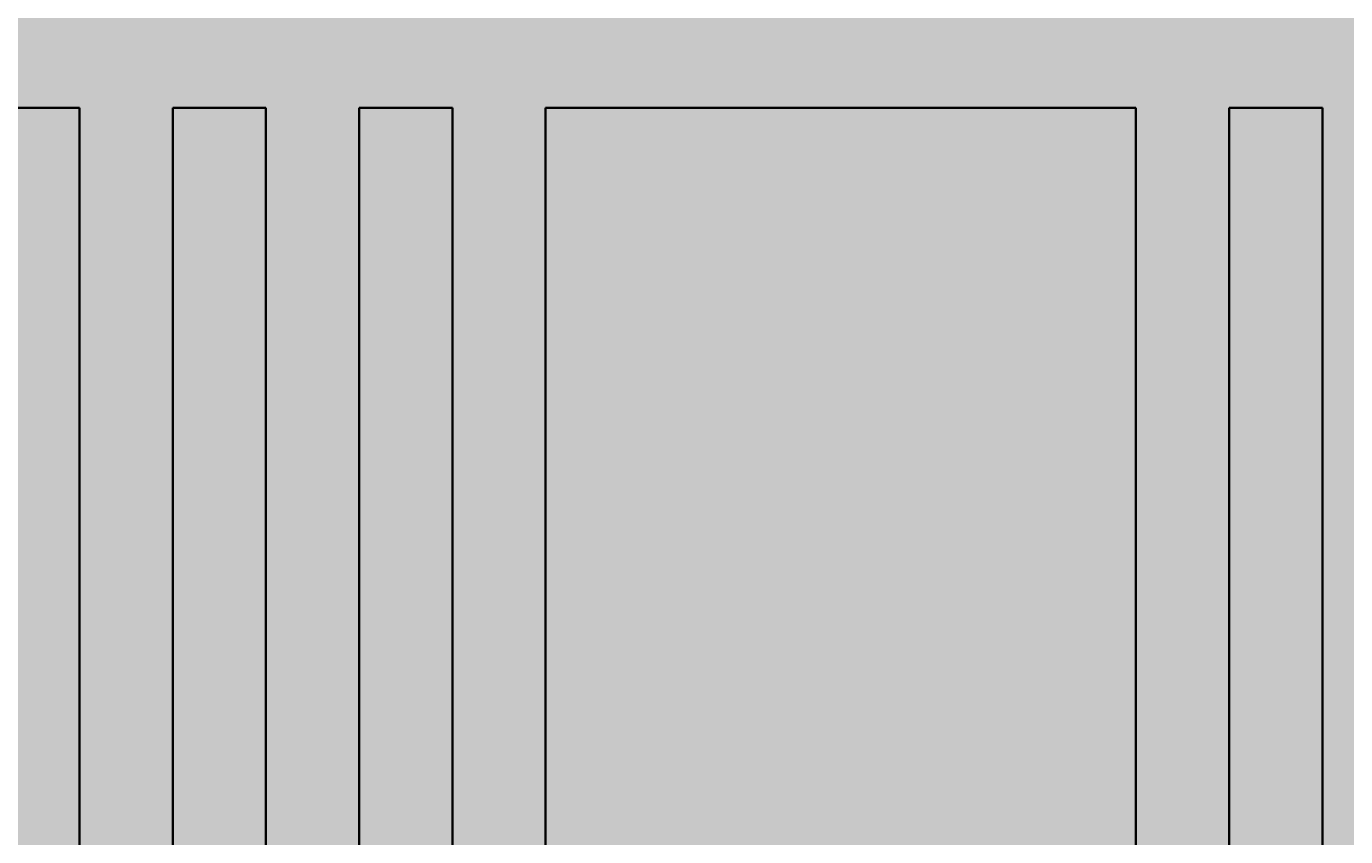
# Model space of a CAD drawing. Units: inches. Extents: x -1 to 292, y -3 to 199.
# Tile 25 of 52: x 106 to 148, y 68 to 95. Entities that reach past the tile are written whole.
import ezdxf

# ---------------------------------------------------------------- set-up
doc = ezdxf.new("R2010")
doc.units = ezdxf.units.IN
doc.header["$MEASUREMENT"] = 0
for name, color, linetype, lineweight in [('M-DIMS', 2, 'Continuous', 18), ('M-EQPM', 7, 'Continuous', 35), ('M-PATT', 8, 'Continuous', 13)]:
    doc.layers.add(name, color=color, linetype=linetype, lineweight=lineweight)
doc.styles.get("Standard").update_dxf_attribs({"font": 'arial.ttf'})
doc.dimstyles.get("Standard").update_dxf_attribs({"dimtxt": 0.18, "dimasz": 0.18, "dimexe": 0.18, "dimexo": 0.0625, "dimgap": 0.09, "dimtad": 0, "dimtih": 1, "dimtoh": 1, "dimdec": 4, "dimzin": 0, "dimdsep": 46, "dimtxsty": 'Standard', "dimcen": 0.09, "dimadec": 0, "dimazin": 0, "dimtfac": 1, "dimtdec": 4, "dimtofl": 0, "dimtmove": 0, "dimatfit": 3, "dimfxl": 1, "dimtolj": 1, "dimtzin": 0, "dimarcsym": 0})

# ---------------------------------------------------------------- blocks, each defined once
blk = doc.blocks.new('BOILER-TUBE')
for p, q in [((0, 40.63), (0, 0)), ((3, 40.63), (3, 0))]:
    blk.add_line(p, q)
for points in [[(0, 40.63), (3, 40.63)], [(3, 0), (0, 0)]]:
    blk.add_lwpolyline(points)
blk = doc.blocks.new('*D8')
at = {"layer": 'Defpoints', "color": 0, "transparency": 16777216}
for p in [(-0.662, 126.765), (111.488, 126.765), (69.013, 25.514)]:
    blk.add_point(p, dxfattribs=at)
at = {"layer": 'M-DIMS', "color": 0, "lineweight": -2, "transparency": 16777216}
for p, q in [((111.426, 126.765), (-0.842, 126.765)), ((-0.662, 126.585), (-0.662, 76.321)), ((-0.662, 25.694), (-0.662, 75.958)), ((68.951, 25.514), (-0.842, 25.514))]:
    blk.add_line(p, q, dxfattribs=at)
at = {"layer": 'M-DIMS', "color": 0, "transparency": 16777216}
for points in [[(-0.692, 126.585), (-0.632, 126.585), (-0.662, 126.765)], [(-0.692, 25.694), (-0.632, 25.694), (-0.662, 25.514)]]:
    blk.add_solid(points, dxfattribs=at)
at = {"layer": 'M-DIMS', "color": 0, "transparency": 16777216, "insert": (-0.662, 76.14), "char_height": 0.18, "attachment_point": 5}
blk.add_mtext('\\A1;101.25', dxfattribs=at)

msp = doc.modelspace()

# ---------------------------------------------------------------- hatches: boundary and pattern name
at = {"layer": 'M-PATT'}
h = msp.add_hatch(color=256, dxfattribs=at)
h.set_gradient(color1=(237, 31, 36), color2=(242, 113, 114), tint=1, name='CYLINDER')
h.paths.add_polyline_path([(106.0735, 105.9941), (106.0735, 106.9941), (108.0603, 106.9941), (107.8488, 107.6501), (57.8007, 107.6501, 0.4142136), (49.9241, 99.7735), (52.3176, 101.3278), (55.0097, 99.7735), (57.4032, 101.3278), (60.0953, 99.7735), (62.4888, 101.3278), (65.1809, 99.7735), (67.5744, 101.3278), (70.2665, 99.7735), (72.66, 101.3278), (75.3521, 99.7735), (77.7456, 101.3278), (80.4377, 99.7735), (82.8312, 101.3278), (85.5233, 99.7735), (87.9168, 101.3278), (90.6089, 99.7735), (93.0024, 101.3278), (95.6945, 99.7735), (98.088, 101.3278), (100.7801, 99.7735), (103.1736, 101.3278), (105.8657, 99.7735), (108.2592, 101.3278), (110.9513, 99.7735), (113.3448, 101.3278), (116.0369, 99.7735), (118.4304, 101.3278), (121.1225, 99.7735), (123.516, 101.3278), (126.2082, 99.7735), (128.6016, 101.3278), (131.2938, 99.7735), (133.6872, 101.3278), (136.3794, 99.7735), (138.7728, 101.3278), (141.465, 99.7735), (143.8584, 101.3278), (146.5506, 99.7735), (148.944, 101.3278), (151.6362, 99.7735), (154.0296, 101.3278), (156.7218, 99.7735), (159.1152, 101.3278), (160.6222, 100.4578), (160.6222, 107.6501), (115.4883, 107.6501), (115.4883, 106.9941), (120.9032, 106.9941), (120.9032, 105.9941), (120.9032, 103.3981), (106.0735, 103.3981)])
h.paths.add_polyline_path([(169.176, 107.6501), (162.1623, 107.6501), (162.1623, 100.004), (164.2008, 101.3278), (166.893, 99.7735), (169.2864, 101.3278), (171.9786, 99.7735), (174.372, 101.3278), (177.0526, 99.7802, 0.4139642)])
h.paths.add_polyline_path([(111.4883, 107.6501), (107.8488, 107.6501), (108.0603, 106.9941), (111.4883, 106.9941)], flags=17)
h.paths.add_polyline_path([(61.6788, 91.897), (57.8007, 91.897, -0.1099266), (54.4604, 92.6403), (43.2011, 92.6403), (23.9502, 84.4688), (23.9502, 58.376), (43.2011, 47.2615), (50.9409, 47.2615, -0.2705926), (57.8007, 51.2672), (61.6788, 51.2672)])
h.paths.add_polyline_path([(73.6788, 91.897), (70.6788, 91.897), (70.6788, 51.2672), (73.6788, 51.2672)])
h.paths.add_polyline_path([(79.6788, 91.897), (76.6788, 91.897), (76.6788, 51.2672), (79.6788, 51.2672)])
h.paths.add_polyline_path([(67.6788, 91.897), (64.6788, 91.897), (64.6788, 51.2672), (67.6788, 51.2672)])
h.paths.add_polyline_path([(101.6788, 91.897), (82.6788, 91.897), (82.6788, 51.2672), (101.6788, 51.2672)])
h.paths.add_polyline_path([(107.6788, 91.897), (104.6788, 91.897), (104.6788, 51.2672), (107.6788, 51.2672)])
h.paths.add_polyline_path([(113.6788, 91.897), (110.6788, 91.897), (110.6788, 51.2672), (113.6788, 51.2672)])
h.paths.add_polyline_path([(119.6788, 91.897), (116.6788, 91.897), (116.6788, 51.2672), (119.6788, 51.2672)])
h.paths.add_polyline_path([(141.6788, 91.897), (122.6788, 91.897), (122.6788, 51.2672), (141.6788, 51.2672)])
h.paths.add_polyline_path([(147.6788, 91.897), (144.6788, 91.897), (144.6788, 51.2672), (147.6788, 51.2672)])
h.paths.add_polyline_path([(153.6788, 91.897), (150.6788, 91.897), (150.6788, 51.2672), (153.6788, 51.2672)])
h.paths.add_polyline_path([(159.6788, 91.897), (156.6788, 91.897), (156.6788, 51.2672), (159.6788, 51.2672)])
h.paths.add_polyline_path([(179.5897, 92.6403), (172.5163, 92.6403, -0.1099266), (169.176, 91.897), (162.6788, 91.897), (162.6788, 51.2672), (169.176, 51.2672, -0.2705926), (176.0358, 47.2615), (179.5897, 47.2615)])
h.paths.add_polyline_path([(203.0265, 84.4688), (183.7755, 92.6403), (181.5897, 92.6403), (181.5897, 47.2615), (183.7755, 47.2615), (203.0265, 58.376)])
h.paths.add_polyline_path([(184.4188, 61.52), (200.7224, 61.52), (200.7224, 77.7532), (184.4188, 77.7532)], flags=24)
h = msp.add_hatch(color=256, dxfattribs=at)
h.set_gradient(color1=(0, 255, 255), color2=(0, 255, 255), tint=1)
h.paths.add_polyline_path([(75.3521, 99.7735), (72.66, 101.3278), (70.2665, 99.7735), (67.5744, 101.3278), (65.1809, 99.7735), (62.4888, 101.3278), (60.0953, 99.7735), (57.4032, 101.3278), (55.0097, 99.7735), (52.3176, 101.3278), (49.9241, 99.7735, 0.4142136), (57.8007, 91.897), (61.6788, 91.897), (61.6788, 51.2672), (57.8007, 51.2672, 0.8088808), (54.5813, 36.2021), (65.0947, 51.2672), (64.6788, 51.2672), (64.6788, 91.897), (67.6788, 91.897), (67.6788, 51.2672), (65.0947, 51.2672), (54.5813, 36.2021, 0.1056561), (57.8007, 35.5141), (169.176, 35.5141, 1), (169.176, 51.2672), (162.6788, 51.2672), (162.6788, 91.897), (169.176, 91.897, 0.4144629), (177.0526, 99.7802), (174.372, 101.3278), (171.9786, 99.7735), (169.2864, 101.3278), (166.893, 99.7735), (164.2008, 101.3278), (162.1623, 100.004), (162.1623, 96.1027), (160.6222, 96.1027), (160.6222, 100.4578), (159.1152, 101.3278), (156.7218, 99.7735), (154.0296, 101.3278), (151.6362, 99.7735), (148.944, 101.3278), (146.5506, 99.7735), (143.8584, 101.3278), (141.465, 99.7735), (138.7728, 101.3278), (136.3794, 99.7735), (133.6872, 101.3278), (131.2938, 99.7735), (128.6016, 101.3278), (126.2082, 99.7735), (123.516, 101.3278), (121.1225, 99.7735), (118.4304, 101.3278), (116.0369, 99.7735), (113.3448, 101.3278), (110.9513, 99.7735), (108.2592, 101.3278), (105.8657, 99.7735), (103.1736, 101.3278), (100.7801, 99.7735), (98.088, 101.3278), (95.6945, 99.7735), (93.0024, 101.3278), (90.6089, 99.7735), (87.9168, 101.3278), (85.5233, 99.7735), (82.8312, 101.3278), (80.4377, 99.7735), (77.7456, 101.3278)])
h.paths.add_polyline_path([(79.6788, 91.897), (79.6788, 51.2672), (76.6788, 51.2672), (76.6788, 91.897)], flags=16)
h.paths.add_polyline_path([(73.6788, 91.897), (73.6788, 51.2672), (70.6788, 51.2672), (70.6788, 91.897)], flags=16)
h.paths.add_polyline_path([(82.6788, 91.897), (101.6788, 91.897), (101.6788, 51.2672), (82.6788, 51.2672)], flags=16)
h.paths.add_polyline_path([(104.6788, 91.897), (107.6788, 91.897), (107.6788, 51.2672), (104.6788, 51.2672)], flags=16)
h.paths.add_polyline_path([(110.6788, 91.897), (113.6788, 91.897), (113.6788, 51.2672), (110.6788, 51.2672)], flags=16)
h.paths.add_polyline_path([(116.6788, 91.897), (119.6788, 91.897), (119.6788, 51.2672), (116.6788, 51.2672)], flags=16)
h.paths.add_polyline_path([(122.6788, 91.897), (141.6788, 91.897), (141.6788, 51.2672), (144.6788, 51.2672), (144.6788, 91.897), (147.6788, 91.897), (147.6788, 51.2672), (122.6788, 51.2672)], flags=16)
h.paths.add_polyline_path([(150.6788, 91.897), (153.6788, 91.897), (153.6788, 51.2672), (150.6788, 51.2672)], flags=16)
h.paths.add_polyline_path([(156.6788, 91.897), (159.6788, 91.897), (159.6788, 51.2672), (156.6788, 51.2672)], flags=16)

# ---------------------------------------------------------------- linework, layer by layer
at = {"layer": 'M-EQPM'}
for p, q in [((122.6788, 91.897), (122.6788, 51.2672)), ((141.6788, 91.897), (141.6788, 51.2672)), ((144.6788, 91.897), (144.6788, 51.2672)), ((147.6788, 91.897), (147.6788, 51.2672))]:
    msp.add_line(p, q, dxfattribs=at)
for points in [[(122.6788, 91.897), (141.6788, 91.897)], [(144.6788, 91.897), (147.6788, 91.897)]]:
    msp.add_lwpolyline(points, dxfattribs=at)

# ---------------------------------------------------------------- block references
for p in [(104.679, 51.267), (110.679, 51.267), (116.679, 51.267)]:
    msp.add_blockref('BOILER-TUBE', p, dxfattribs=at)

# ---------------------------------------------------------------- dimensions: what is measured, and where the dimension line sits
at = {"layer": 'M-DIMS'}
dim = msp.add_linear_dim(base=(-0.6625, 126.765), p1=(69.013, 25.5141), p2=(111.4883, 126.765), angle=90, dimstyle='Standard', override={"dimdec": 2, "dimlfac": 1, "dimrnd": 0, "dimzin": 0, "dimdsep": 46, "dimlunit": 2}, dxfattribs=at)
dim.commit()
dim.dimension.update_dxf_attribs({"geometry": '*D8', "text_midpoint": (-0.6625, 76.1396)})

doc.saveas('drawing.dxf')
